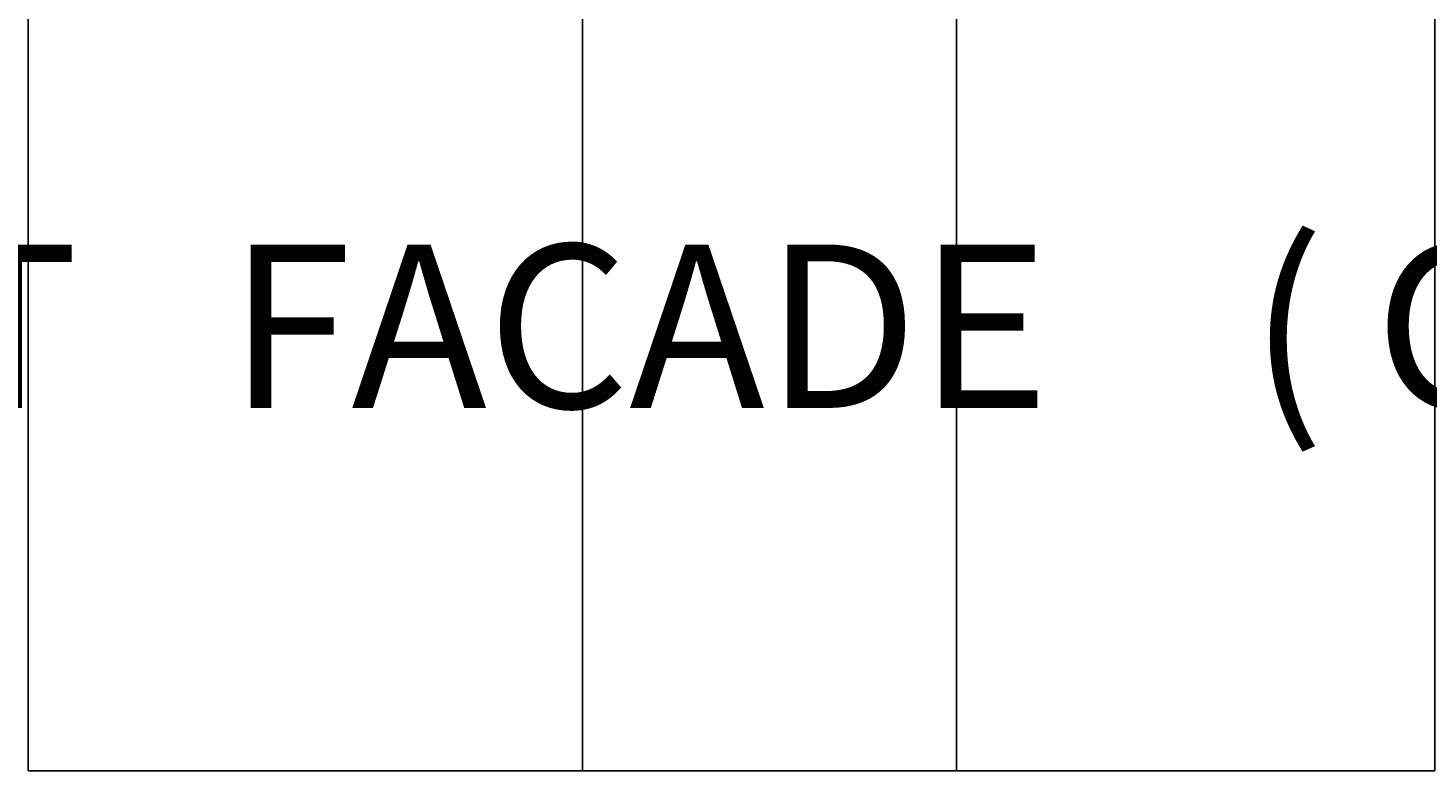
# Model space of a CAD drawing. Units: inches. Extents: x -32109 to 33221, y -19197 to 7608.
# Tile 9 of 25: x -11787 to -5707, y -5430 to -2204. Entities that reach past the tile are written whole.
import ezdxf

# ---------------------------------------------------------------- set-up
doc = ezdxf.new("R2010")
doc.units = ezdxf.units.IN
doc.header["$MEASUREMENT"] = 0
doc.layers.add('A-ANNO-DIMS', color=2, linetype='Continuous', lineweight=18)
doc.layers.add('A-ANNO-TEXT', color=7, linetype='Continuous', lineweight=25)
doc.styles.get("Standard").update_dxf_attribs({"font": 'arial.ttf'})
doc.dimstyles.get("Standard").update_dxf_attribs({"dimtxt": 0.18, "dimasz": 0.18, "dimexe": 0.18, "dimexo": 0.0625, "dimgap": 0.09, "dimtad": 0, "dimtih": 1, "dimtoh": 1, "dimdec": 4, "dimzin": 0, "dimdsep": 46, "dimtxsty": 'Standard', "dimcen": 0.09, "dimadec": 0, "dimazin": 0, "dimtfac": 1, "dimtdec": 4, "dimtofl": 0, "dimtmove": 0, "dimatfit": 3, "dimfxl": 1, "dimtolj": 1, "dimtzin": 0, "dimarcsym": 0})

# ---------------------------------------------------------------- blocks, each defined once
blk = doc.blocks.new('*D27')
at = {"layer": 'A-ANNO-DIMS', "color": 0, "lineweight": -2, "transparency": 16777216}
for p, q in [((-11787, -2124.9), (-11787, -5429.7)), ((-9378.4, -2124.9), (-9378.4, -5429.7)), ((-11786.8, -5429.6), (-10583.2, -5429.6)), ((-9378.6, -5429.6), (-10582.2, -5429.6))]:
    blk.add_line(p, q, dxfattribs=at)
at = {"layer": 'A-ANNO-DIMS', "color": 0, "transparency": 16777216}
for points in [[(-11786.8, -5429.5), (-11786.8, -5429.6), (-11787, -5429.6)], [(-9378.6, -5429.5), (-9378.6, -5429.6), (-9378.4, -5429.6)]]:
    blk.add_solid(points, dxfattribs=at)
at = {"layer": 'Defpoints', "color": 0, "transparency": 16777216}
for p in [(-11787, -2124.8), (-9378.4, -2124.8), (-9378.4, -5429.6)]:
    blk.add_point(p, dxfattribs=at)
at = {"layer": 'A-ANNO-DIMS', "color": 0, "transparency": 16777216, "insert": (-10582.7, -5429.6), "char_height": 0.18, "attachment_point": 5}
blk.add_mtext('\\A1;2408.6', dxfattribs=at)
blk = doc.blocks.new('*D28')
at = {"layer": 'A-ANNO-DIMS', "color": 0, "lineweight": -2, "transparency": 16777216}
for p, q in [((-9378.4, -2124.9), (-9378.4, -5429.7)), ((-7754.4, -2118.5), (-7754.4, -5429.7)), ((-9378.2, -5429.6), (-8566.7, -5429.6)), ((-7754.6, -5429.6), (-8566, -5429.6))]:
    blk.add_line(p, q, dxfattribs=at)
at = {"layer": 'A-ANNO-DIMS', "color": 0, "transparency": 16777216}
for points in [[(-9378.2, -5429.5), (-9378.2, -5429.6), (-9378.4, -5429.6)], [(-7754.6, -5429.5), (-7754.6, -5429.6), (-7754.4, -5429.6)]]:
    blk.add_solid(points, dxfattribs=at)
at = {"layer": 'Defpoints', "color": 0, "transparency": 16777216}
for p in [(-9378.4, -2124.8), (-7754.4, -2118.4), (-7754.4, -5429.6)]:
    blk.add_point(p, dxfattribs=at)
at = {"layer": 'A-ANNO-DIMS', "color": 0, "transparency": 16777216, "insert": (-8566.4, -5429.6), "char_height": 0.18, "attachment_point": 5}
blk.add_mtext('\\A1;1624', dxfattribs=at)
blk = doc.blocks.new('*D29')
at = {"layer": 'A-ANNO-DIMS', "color": 0, "lineweight": -2, "transparency": 16777216}
for p, q in [((-7754.4, -2118.5), (-7754.4, -5429.7)), ((-5677.1, -2124.9), (-5677.1, -5429.7)), ((-7754.2, -5429.6), (-6716.2, -5429.6)), ((-5677.3, -5429.6), (-6715.3, -5429.6))]:
    blk.add_line(p, q, dxfattribs=at)
at = {"layer": 'A-ANNO-DIMS', "color": 0, "transparency": 16777216}
for points in [[(-7754.2, -5429.5), (-7754.2, -5429.6), (-7754.4, -5429.6)], [(-5677.3, -5429.5), (-5677.3, -5429.6), (-5677.1, -5429.6)]]:
    blk.add_solid(points, dxfattribs=at)
at = {"layer": 'Defpoints', "color": 0, "transparency": 16777216}
for p in [(-7754.4, -2118.4), (-5677.1, -2124.8), (-5677.1, -5429.6)]:
    blk.add_point(p, dxfattribs=at)
at = {"layer": 'A-ANNO-DIMS', "color": 0, "transparency": 16777216, "insert": (-6715.7, -5429.6), "char_height": 0.18, "attachment_point": 5}
blk.add_mtext('\\A1;2077.3', dxfattribs=at)

msp = doc.modelspace()

# ---------------------------------------------------------------- texts
at = {"layer": 'A-ANNO-TEXT'}
msp.add_text('MONUMENTAL    FRONT   FACADE    ( CONCEPTUAL ONLY   NO DIMENSIONS )', height=709.79495, dxfattribs=at).set_placement((-22238.107, -3853.852))

# ---------------------------------------------------------------- dimensions: what is measured, and where the dimension line sits
at = {"layer": 'A-ANNO-DIMS'}
for base, p1, p2, override, picture, middle in [((-9378.383, -5429.555), (-11787.012, -2124.791), (-9378.383, -2124.791), {"dimdec": 1, "dimlfac": 1, "dimrnd": 0, "dimzin": 0, "dimdsep": 46, "dimlunit": 2}, '*D27', (-10582.697, -5429.555)), ((-7754.412, -5429.555), (-9378.383, -2124.791), (-7754.412, -2118.431), {"dimdec": 0, "dimlfac": 1, "dimrnd": 0, "dimzin": 0, "dimdsep": 46, "dimlunit": 2}, '*D28', (-8566.398, -5429.555)), ((-5677.079, -5429.555), (-7754.412, -2118.431), (-5677.079, -2124.791), {"dimdec": 1, "dimlfac": 1, "dimrnd": 0, "dimzin": 0, "dimdsep": 46, "dimlunit": 2}, '*D29', (-6715.746, -5429.555))]:
    dim = msp.add_linear_dim(base=base, p1=p1, p2=p2, dimstyle='Standard', override=override, dxfattribs=at)
    dim.commit()
    dim.dimension.update_dxf_attribs({"geometry": picture, "text_midpoint": middle})

doc.saveas('drawing.dxf')
